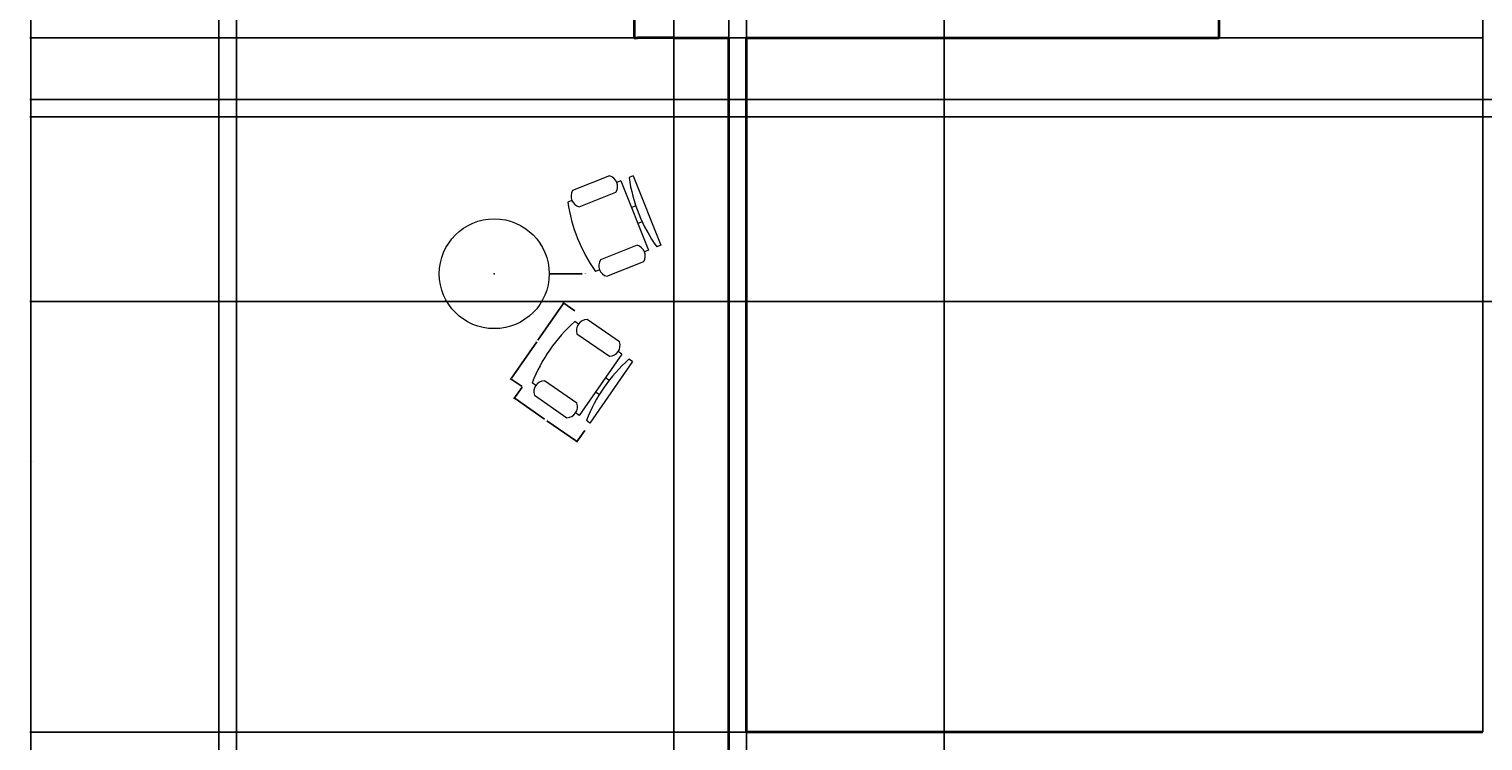
# Model space of a CAD drawing. Units: inches. Extents: x 2024 to 2965, y 1692 to 2308.
# Tile 2 of 8: x 2024 to 2355, y 1972 to 2134. Entities that reach past the tile are written whole.
import ezdxf

# ---------------------------------------------------------------- set-up
doc = ezdxf.new("R2010")
doc.units = ezdxf.units.IN
for name, color, linetype, lineweight in [('A-ANNO-DIMS', 2, 'Continuous', 18), ('A-FLOR-OTLN', 7, 'Continuous', 25), ('A-FURN', 8, 'Continuous', 18), ('A-WALL', 7, 'Continuous', 35)]:
    doc.layers.add(name, color=color, linetype=linetype, lineweight=lineweight)
doc.styles.get("Standard").update_dxf_attribs({"font": 'arial.ttf'})
doc.dimstyles.get("Standard").update_dxf_attribs({"dimtxt": 0.18, "dimasz": 0.18, "dimexe": 0.18, "dimexo": 0.0625, "dimgap": 0.09, "dimtad": 0, "dimtih": 1, "dimtoh": 1, "dimdec": 4, "dimzin": 0, "dimdsep": 46, "dimtxsty": 'Standard', "dimcen": 0.09, "dimadec": 0, "dimazin": 0, "dimtfac": 1, "dimtdec": 4, "dimtofl": 0, "dimtmove": 0, "dimatfit": 3, "dimfxl": 1, "dimtolj": 1, "dimtzin": 0, "dimarcsym": 0})

# ---------------------------------------------------------------- blocks, each defined once
blk = doc.blocks.new('Chair - Desk')
for p, q in [((-8.5, 0), (-8.5, -1)), ((-8.5, 0), (8.5, 0)), ((8.5, 0), (8.5, -1)), ((-8.5, -3), (-8.5, -4)), ((-8.5, -3), (8.5, -3)), ((-2, -3), (-2, -1.9355)), ((2, -1.9576), (2, -3)), ((8.5, -3), (8.5, -4)), ((-10.5, -5), (-10.5, -14)), ((-6.5, -14), (-6.5, -5)), ((6.5, -5), (6.5, -14)), ((10.5, -14), (10.5, -5)), ((-8.5, -15), (-8.5, -16)), ((8.5, -15), (8.5, -16))]:
    blk.add_line(p, q)
for centre, radius, start, end in [((0, 34.625), 36.625, 256.5803, 283.4197), ((-8.5, -6.5), 2.5, 36.8699, 143.1301), ((8.5, -6.5), 2.5, 36.8699, 143.1301), ((-8.5, -12.5), 2.5, 216.8699, 323.1301), ((0, 19.625), 36.625, 256.5803, 283.4197), ((8.5, -12.5), 2.5, 216.8699, 323.1301)]:
    blk.add_arc(centre, radius, start, end)
blk = doc.blocks.new('*D49')
at = {"layer": 'A-ANNO-DIMS', "color": 0, "lineweight": -2, "transparency": 16777216}
for p, q in [((2145.75, 2071.26), (2140, 2062.97)), ((2148.39, 2069.65), (2145.71, 2071.51)), ((2133.99, 2054.31), (2139.74, 2062.6)), ((2136.42, 2052.4), (2133.74, 2054.26))]:
    blk.add_line(p, q, dxfattribs=at)
at = {"layer": 'A-ANNO-DIMS', "color": 0, "transparency": 16777216}
for points in [[(2145.73, 2071.28), (2145.78, 2071.25), (2145.86, 2071.41)], [(2133.96, 2054.32), (2134.01, 2054.29), (2133.88, 2054.16)]]:
    blk.add_solid(points, dxfattribs=at)
at = {"layer": 'Defpoints', "color": 0, "transparency": 16777216}
for p in [(2148.45, 2069.62), (2133.88, 2054.16), (2136.47, 2052.36)]:
    blk.add_point(p, dxfattribs=at)
at = {"layer": 'A-ANNO-DIMS', "color": 0, "transparency": 16777216, "insert": (2139.87, 2062.79), "char_height": 0.18, "attachment_point": 5}
blk.add_mtext('\\A1;CHAIR 21 TYP.', dxfattribs=at)
blk = doc.blocks.new('*D50')
at = {"layer": 'A-ANNO-DIMS', "color": 0, "lineweight": -2, "transparency": 16777216}
for p, q in [((2136.44, 2052.31), (2134.57, 2049.63)), ((2134.82, 2049.67), (2141.54, 2045.01)), ((2148.77, 2040), (2142.06, 2044.65)), ((2150.68, 2042.43), (2148.81, 2039.74))]:
    blk.add_line(p, q, dxfattribs=at)
at = {"layer": 'A-ANNO-DIMS', "color": 0, "transparency": 16777216}
for points in [[(2134.84, 2049.7), (2134.81, 2049.65), (2134.68, 2049.78)], [(2148.79, 2040.02), (2148.75, 2039.97), (2148.92, 2039.89)]]:
    blk.add_solid(points, dxfattribs=at)
at = {"layer": 'Defpoints', "color": 0, "transparency": 16777216}
for p in [(2136.47, 2052.36), (2148.92, 2039.89), (2150.71, 2042.48)]:
    blk.add_point(p, dxfattribs=at)
at = {"layer": 'A-ANNO-DIMS', "color": 0, "transparency": 16777216, "insert": (2141.8, 2044.83), "char_height": 0.18, "attachment_point": 5}
blk.add_mtext('\\A1;17 TYP.', dxfattribs=at)
blk = doc.blocks.new('*D84')
at = {"layer": 'A-ANNO-DIMS', "color": 0, "lineweight": -2, "transparency": 16777216}
for p, q in [((2618.84, 2255.77), (2024.5, 2255.77)), ((2024.68, 2255.59), (2024.68, 2163.96)), ((2024.68, 2071.95), (2024.68, 2163.59)), ((2618.84, 2071.77), (2024.5, 2071.77))]:
    blk.add_line(p, q, dxfattribs=at)
at = {"layer": 'A-ANNO-DIMS', "color": 0, "transparency": 16777216}
for points in [[(2024.65, 2255.59), (2024.71, 2255.59), (2024.68, 2255.77)], [(2024.65, 2071.95), (2024.71, 2071.95), (2024.68, 2071.77)]]:
    blk.add_solid(points, dxfattribs=at)
at = {"layer": 'Defpoints', "color": 0, "transparency": 16777216}
for p in [(2024.68, 2255.77), (2618.91, 2255.77), (2618.91, 2071.77)]:
    blk.add_point(p, dxfattribs=at)
at = {"layer": 'A-ANNO-DIMS', "color": 0, "transparency": 16777216, "insert": (2024.68, 2163.77), "char_height": 0.18, "attachment_point": 5}
blk.add_mtext('\\A1;184', dxfattribs=at)
blk = doc.blocks.new('*D88')
at = {"layer": 'A-ANNO-DIMS', "color": 0, "lineweight": -2, "transparency": 16777216}
for p, q in [((2817.84, 2260.77), (2024.5, 2260.77)), ((2024.68, 2260.59), (2024.68, 2189.46)), ((2024.68, 2117.95), (2024.68, 2189.09)), ((2817.84, 2117.77), (2024.5, 2117.77))]:
    blk.add_line(p, q, dxfattribs=at)
at = {"layer": 'A-ANNO-DIMS', "color": 0, "transparency": 16777216}
for points in [[(2024.65, 2260.59), (2024.71, 2260.59), (2024.68, 2260.77)], [(2024.65, 2117.95), (2024.71, 2117.95), (2024.68, 2117.77)]]:
    blk.add_solid(points, dxfattribs=at)
at = {"layer": 'Defpoints', "color": 0, "transparency": 16777216}
for p in [(2817.91, 2260.77), (2024.68, 2117.77), (2817.91, 2117.77)]:
    blk.add_point(p, dxfattribs=at)
at = {"layer": 'A-ANNO-DIMS', "color": 0, "transparency": 16777216, "insert": (2024.68, 2189.27), "char_height": 0.18, "attachment_point": 5}
blk.add_mtext('\\A1;143', dxfattribs=at)
blk = doc.blocks.new('*D90')
at = {"layer": 'A-ANNO-DIMS', "color": 0, "lineweight": -2, "transparency": 16777216}
for p, q in [((2067.4, 2148.35), (2024.5, 2148.35)), ((2024.68, 2148.17), (2024.68, 2040.53)), ((2024.68, 1932.53), (2024.68, 2040.17)), ((2067.4, 1932.35), (2024.5, 1932.35))]:
    blk.add_line(p, q, dxfattribs=at)
at = {"layer": 'A-ANNO-DIMS', "color": 0, "transparency": 16777216}
for points in [[(2024.65, 2148.17), (2024.71, 2148.17), (2024.68, 2148.35)], [(2024.65, 1932.53), (2024.71, 1932.53), (2024.68, 1932.35)]]:
    blk.add_solid(points, dxfattribs=at)
at = {"layer": 'Defpoints', "color": 0, "transparency": 16777216}
for p in [(2024.68, 2148.35), (2067.46, 2148.35), (2067.46, 1932.35)]:
    blk.add_point(p, dxfattribs=at)
at = {"layer": 'A-ANNO-DIMS', "color": 0, "transparency": 16777216, "insert": (2024.68, 2040.35), "char_height": 0.18, "attachment_point": 5}
blk.add_mtext('\\A1;216', dxfattribs=at)
blk = doc.blocks.new('*D91')
at = {"layer": 'A-ANNO-DIMS', "color": 0, "lineweight": -2, "transparency": 16777216}
for p, q in [((2071.46, 1936.41), (2071.46, 2307.73)), ((2183.46, 1936.41), (2183.46, 2307.73)), ((2071.64, 2307.55), (2127.18, 2307.55)), ((2183.28, 2307.55), (2127.74, 2307.55))]:
    blk.add_line(p, q, dxfattribs=at)
at = {"layer": 'A-ANNO-DIMS', "color": 0, "transparency": 16777216}
for points in [[(2071.64, 2307.58), (2071.64, 2307.52), (2071.46, 2307.55)], [(2183.28, 2307.58), (2183.28, 2307.52), (2183.46, 2307.55)]]:
    blk.add_solid(points, dxfattribs=at)
at = {"layer": 'Defpoints', "color": 0, "transparency": 16777216}
for p in [(2183.46, 2307.55), (2071.46, 1936.35), (2183.46, 1936.35)]:
    blk.add_point(p, dxfattribs=at)
at = {"layer": 'A-ANNO-DIMS', "color": 0, "transparency": 16777216, "insert": (2127.46, 2307.55), "char_height": 0.18, "attachment_point": 5}
blk.add_mtext('\\A1;112', dxfattribs=at)
blk = doc.blocks.new('*D93')
at = {"layer": 'A-ANNO-DIMS', "color": 0, "lineweight": -2, "transparency": 16777216}
for p, q in [((2187.46, 1932.41), (2187.46, 2307.73)), ((2418.91, 1933.84), (2418.91, 2307.73)), ((2187.64, 2307.55), (2302.72, 2307.55)), ((2418.73, 2307.55), (2303.65, 2307.55))]:
    blk.add_line(p, q, dxfattribs=at)
at = {"layer": 'A-ANNO-DIMS', "color": 0, "transparency": 16777216}
for points in [[(2187.64, 2307.58), (2187.64, 2307.52), (2187.46, 2307.55)], [(2418.73, 2307.58), (2418.73, 2307.52), (2418.91, 2307.55)]]:
    blk.add_solid(points, dxfattribs=at)
at = {"layer": 'Defpoints', "color": 0, "transparency": 16777216}
for p in [(2418.91, 2307.55), (2187.46, 1932.35), (2418.91, 1933.77)]:
    blk.add_point(p, dxfattribs=at)
at = {"layer": 'A-ANNO-DIMS', "color": 0, "transparency": 16777216, "insert": (2303.18, 2307.55), "char_height": 0.18, "attachment_point": 5}
blk.add_mtext('\\A1;231.45', dxfattribs=at)
blk = doc.blocks.new('*D94')
at = {"layer": 'A-ANNO-DIMS', "color": 0, "lineweight": -2, "transparency": 16777216}
for p, q in [((2187.46, 1973.84), (2187.46, 2307.73)), ((2354.91, 1973.84), (2354.91, 2307.73)), ((2187.64, 2307.55), (2270.73, 2307.55)), ((2354.73, 2307.55), (2271.64, 2307.55))]:
    blk.add_line(p, q, dxfattribs=at)
at = {"layer": 'A-ANNO-DIMS', "color": 0, "transparency": 16777216}
for points in [[(2187.64, 2307.58), (2187.64, 2307.52), (2187.46, 2307.55)], [(2354.73, 2307.58), (2354.73, 2307.52), (2354.91, 2307.55)]]:
    blk.add_solid(points, dxfattribs=at)
at = {"layer": 'Defpoints', "color": 0, "transparency": 16777216}
for p in [(2354.91, 2307.55), (2187.46, 1973.77), (2354.91, 1973.77)]:
    blk.add_point(p, dxfattribs=at)
at = {"layer": 'A-ANNO-DIMS', "color": 0, "transparency": 16777216, "insert": (2271.18, 2307.55), "char_height": 0.18, "attachment_point": 5}
blk.add_mtext('\\A1;167.45', dxfattribs=at)
blk = doc.blocks.new('*D95')
at = {"layer": 'A-ANNO-DIMS', "color": 0, "lineweight": -2, "transparency": 16777216}
for p, q in [((2354.84, 2131.77), (2024.5, 2131.77)), ((2024.68, 2131.59), (2024.68, 2052.96)), ((2024.68, 1973.95), (2024.68, 2052.59)), ((2354.84, 1973.77), (2024.5, 1973.77))]:
    blk.add_line(p, q, dxfattribs=at)
at = {"layer": 'A-ANNO-DIMS', "color": 0, "transparency": 16777216}
for points in [[(2024.65, 2131.59), (2024.71, 2131.59), (2024.68, 2131.77)], [(2024.65, 1973.95), (2024.71, 1973.95), (2024.68, 1973.77)]]:
    blk.add_solid(points, dxfattribs=at)
at = {"layer": 'Defpoints', "color": 0, "transparency": 16777216}
for p in [(2024.68, 2131.77), (2354.91, 2131.77), (2354.91, 1973.77)]:
    blk.add_point(p, dxfattribs=at)
at = {"layer": 'A-ANNO-DIMS', "color": 0, "transparency": 16777216, "insert": (2024.68, 2052.77), "char_height": 0.18, "attachment_point": 5}
blk.add_mtext('\\A1;158', dxfattribs=at)
blk = doc.blocks.new('*D101')
at = {"layer": 'A-ANNO-DIMS', "color": 0, "lineweight": -2, "transparency": 16777216}
for p, q in [((2917.96, 2113.77), (2024.5, 2113.77)), ((2024.68, 2113.59), (2024.68, 2035.52)), ((2024.68, 1957.09), (2024.68, 2035.16)), ((2917.96, 1956.91), (2024.5, 1956.91))]:
    blk.add_line(p, q, dxfattribs=at)
at = {"layer": 'A-ANNO-DIMS', "color": 0, "transparency": 16777216}
for points in [[(2024.65, 2113.59), (2024.71, 2113.59), (2024.68, 2113.77)], [(2024.65, 1957.09), (2024.71, 1957.09), (2024.68, 1956.91)]]:
    blk.add_solid(points, dxfattribs=at)
at = {"layer": 'Defpoints', "color": 0, "transparency": 16777216}
for p in [(2024.68, 2113.77), (2918.02, 2113.77), (2918.02, 1956.91)]:
    blk.add_point(p, dxfattribs=at)
at = {"layer": 'A-ANNO-DIMS', "color": 0, "transparency": 16777216, "insert": (2024.68, 2035.34), "char_height": 0.18, "attachment_point": 5}
blk.add_mtext('\\A1;156.87', dxfattribs=at)
blk = doc.blocks.new('*D116')
at = {"layer": 'A-ANNO-DIMS', "color": 0, "lineweight": -2, "transparency": 16777216}
for p, q in [((2170.91, 1793.84), (2170.91, 2307.73)), ((2232.43, 1793.84), (2232.43, 2307.73)), ((2171.09, 2307.55), (2201.27, 2307.55)), ((2232.25, 2307.55), (2202.06, 2307.55))]:
    blk.add_line(p, q, dxfattribs=at)
at = {"layer": 'A-ANNO-DIMS', "color": 0, "transparency": 16777216}
for points in [[(2171.09, 2307.58), (2171.09, 2307.52), (2170.91, 2307.55)], [(2232.25, 2307.58), (2232.25, 2307.52), (2232.43, 2307.55)]]:
    blk.add_solid(points, dxfattribs=at)
at = {"layer": 'Defpoints', "color": 0, "transparency": 16777216}
for p in [(2232.43, 2307.55), (2170.91, 1793.77), (2232.43, 1793.77)]:
    blk.add_point(p, dxfattribs=at)
at = {"layer": 'A-ANNO-DIMS', "color": 0, "transparency": 16777216, "insert": (2201.67, 2307.55), "char_height": 0.18, "attachment_point": 5}
blk.add_mtext('\\A1;61.52', dxfattribs=at)
blk = doc.blocks.new('*D119')
at = {"layer": 'A-ANNO-DIMS', "color": 0, "lineweight": -2, "transparency": 16777216}
for p, q in [((2130, 2078.09), (2130.18, 2078.09)), ((2130.09, 2078), (2130.09, 2078.18)), ((2150.09, 2078.09), (2142.77, 2078.09))]:
    blk.add_line(p, q, dxfattribs=at)
at = {"layer": 'A-ANNO-DIMS', "color": 0, "transparency": 16777216}
blk.add_solid([(2142.77, 2078.12), (2142.77, 2078.06), (2142.59, 2078.09)], dxfattribs=at)
at = {"layer": 'Defpoints', "color": 0, "transparency": 16777216}
for p in [(2117.6, 2078.09), (2142.59, 2078.09)]:
    blk.add_point(p, dxfattribs=at)
at = {"layer": 'A-ANNO-DIMS', "color": 0, "transparency": 16777216, "insert": (2150.65, 2078.09), "char_height": 0.18, "attachment_point": 5}
blk.add_mtext('\\A1;∅24.993', dxfattribs=at)

msp = doc.modelspace()

# ---------------------------------------------------------------- linework, layer by layer
at = {"layer": 'A-FLOR-OTLN'}
for points in [[(2161.9061, 2148.352), (2067.4594, 2148.352), (2067.4594, 1932.352), (2161.9061, 1932.352)], [(2161.9061, 2144.352), (2071.4594, 2144.352), (2071.4594, 1936.352), (2170.9061, 1936.352)]]:
    msp.add_lwpolyline(points, dxfattribs=at)
at = {"layer": 'A-FURN'}
msp.add_circle((2130.0917, 2078.0928), 12.4965, dxfattribs=at)
at = {"layer": 'A-WALL'}
for p, q in [((2161.9061, 2144.352), (2161.9061, 2131.7595)), ((2294.9061, 2131.7736), (2294.9061, 2141.7736)), ((2161.9061, 2131.7595), (2162.6552, 2131.7736)), ((2170.9061, 2131.7736), (2162.6552, 2131.7736)), ((2170.9061, 2131.7736), (2183.4594, 2131.7736)), ((2187.4594, 2131.7736), (2294.9061, 2131.7736)), ((2354.9061, 1973.7736), (2187.4594, 1973.7736))]:
    msp.add_line(p, q, dxfattribs=at)
for points in [[(2183.4594, 1973.7736), (2183.4594, 2131.7736)], [(2183.4594, 1969.7736), (2183.4594, 2131.7736)], [(2187.4594, 1973.7736), (2187.4594, 2131.7736)]]:
    msp.add_lwpolyline(points, dxfattribs=at)

# ---------------------------------------------------------------- block references
at = {"layer": 'A-FURN'}
for p, rotation in [((2164.817, 2092.46), 291.8014094863518), ((2156.6992, 2051.107), 235.2405251970198)]:
    msp.add_blockref('Chair - Desk', p, dxfattribs=dict(at, rotation=rotation))

# ---------------------------------------------------------------- dimensions: what is measured, and where the dimension line sits
at = {"layer": 'A-ANNO-DIMS'}
for base, p1, p2, override, picture, middle in [((2183.4594, 2307.5486), (2071.4594, 1936.352), (2183.4594, 1936.352), {"dimdec": 0, "dimlfac": 1, "dimrnd": 0, "dimzin": 0, "dimdsep": 46, "dimlunit": 2}, '*D91', (2127.4594, 2307.5486)), ((2232.4289, 2307.5486), (2170.9061, 1793.7736), (2232.4289, 1793.7736), {"dimdec": 2, "dimlfac": 1, "dimrnd": 0, "dimzin": 0, "dimdsep": 46, "dimlunit": 2}, '*D116', (2201.6675, 2307.5486)), ((2418.9061, 2307.5486), (2187.4594, 1932.352), (2418.9061, 1933.7736), {"dimdec": 2, "dimlfac": 1, "dimrnd": 0, "dimzin": 0, "dimdsep": 46, "dimlunit": 2}, '*D93', (2303.1828, 2307.5486)), ((2354.9061, 2307.5486), (2187.4594, 1973.7736), (2354.9061, 1973.7736), {"dimdec": 2, "dimlfac": 1, "dimrnd": 0, "dimzin": 0, "dimdsep": 46, "dimlunit": 2}, '*D94', (2271.1828, 2307.5486))]:
    dim = msp.add_linear_dim(base=base, p1=p1, p2=p2, dimstyle='Standard', override=override, dxfattribs=at)
    dim.commit()
    dim.dimension.update_dxf_attribs({"geometry": picture, "text_midpoint": middle})
for base, p1, p2, override, picture, middle in [((2024.6844, 2117.7736), (2817.9061, 2260.7736), (2817.9061, 2117.7736), {"dimdec": 0, "dimlfac": 1, "dimrnd": 0, "dimzin": 0, "dimdsep": 46, "dimlunit": 2}, '*D88', (2024.6844, 2189.2736)), ((2024.6844, 2255.7736), (2618.9061, 2071.7736), (2618.9061, 2255.7736), {"dimdec": 0, "dimlfac": 1, "dimrnd": 0, "dimzin": 0, "dimdsep": 46, "dimlunit": 2}, '*D84', (2024.6844, 2163.7736)), ((2024.6844, 2148.352), (2067.4594, 1932.352), (2067.4594, 2148.352), {"dimdec": 0, "dimlfac": 1, "dimrnd": 0, "dimzin": 0, "dimdsep": 46, "dimlunit": 2}, '*D90', (2024.6844, 2040.352)), ((2024.6844, 2131.7736), (2354.9061, 1973.7736), (2354.9061, 2131.7736), {"dimdec": 0, "dimlfac": 1, "dimrnd": 0, "dimzin": 0, "dimdsep": 46, "dimlunit": 2}, '*D95', (2024.6844, 2052.7736)), ((2024.6844, 2113.7736), (2918.0192, 1956.9082), (2918.0192, 2113.7736), {"dimdec": 2, "dimlfac": 1, "dimrnd": 0, "dimzin": 0, "dimdsep": 46, "dimlunit": 2}, '*D101', (2024.6844, 2035.3409))]:
    dim = msp.add_linear_dim(base=base, p1=p1, p2=p2, angle=90, dimstyle='Standard', override=override, dxfattribs=at)
    dim.commit()
    dim.dimension.update_dxf_attribs({"geometry": picture, "text_midpoint": middle})
dim = msp.add_diameter_dim_2p(p1=(2117.5952, 2078.0926), p2=(2142.5882, 2078.093), dimstyle='Standard', override={"dimdec": 3, "dimlfac": 1, "dimrnd": 0, "dimzin": 0, "dimdsep": 46, "dimlunit": 2}, dxfattribs=at)
dim.commit()
dim.dimension.update_dxf_attribs({"geometry": '*D119', "text_midpoint": (2150.0861, 2078.0931), "dimtype": 163})
for base, p1, p2, angle, text, picture, middle in [((2133.8846, 2054.1589), (2148.4453, 2069.6156), (2136.4725, 2052.363), 235.240525, 'CHAIR <> TYP.', '*D49', (2139.871, 2062.7852)), ((2148.9168, 2039.8928), (2136.4725, 2052.363), (2150.7128, 2042.4807), 325.240525, '<> TYP.', '*D50', (2141.7967, 2044.8339))]:
    dim = msp.add_linear_dim(base=base, p1=p1, p2=p2, angle=angle, text=text, dimstyle='Standard', override={"dimdec": 0, "dimlfac": 1, "dimrnd": 0, "dimzin": 0, "dimdsep": 46, "dimlunit": 2}, dxfattribs=at)
    dim.commit()
    dim.dimension.update_dxf_attribs({"geometry": picture, "text_midpoint": middle})

doc.saveas('drawing.dxf')
